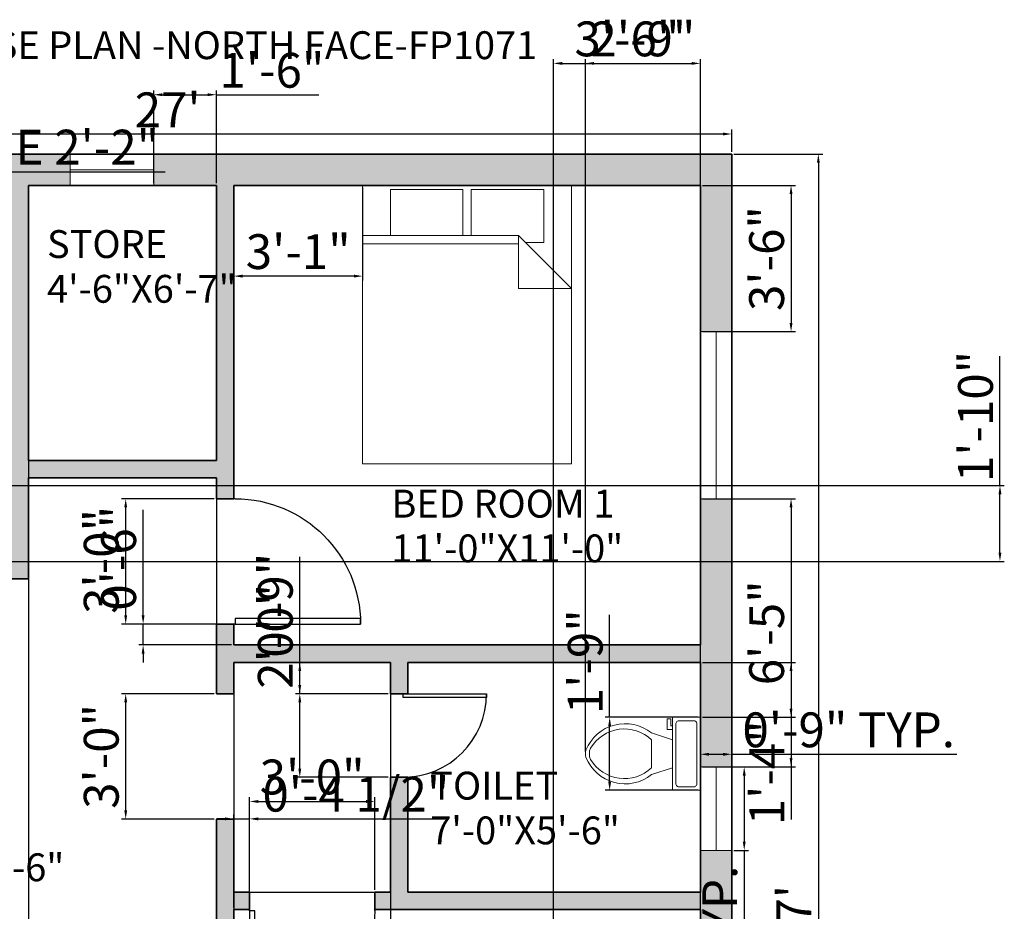
# Model space of a CAD drawing. Units: inches. Extents: x 3647 to 4124, y 1633 to 2205.
# Tile 3 of 3: x 3833 to 4116, y 1919 to 2175. Entities that reach past the tile are written whole.
import ezdxf

# ---------------------------------------------------------------- set-up
doc = ezdxf.new("R2010")
doc.units = ezdxf.units.IN
for name, color, linetype, lineweight in [('A-ANNO-DIMS', 2, 'Continuous', 18), ('A-ANNO-TEXT', 3, 'Continuous', 25), ('A-AREA-IDEN', 3, 'Continuous', 18), ('A-FLOR-FIXT', 9, 'Continuous', 18), ('A-FURN', 8, 'Continuous', 18), ('DOOR', 6, 'Continuous', 25), ('WALL', 42, 'Continuous', 35), ('WINDOW', 4, 'Continuous', 18)]:
    doc.layers.add(name, color=color, linetype=linetype, lineweight=lineweight)
doc.layers.add('A-WALL-PATT', color=18, linetype='Continuous', lineweight=13, true_color=0x000000)
doc.styles.get("Standard").update_dxf_attribs({"font": 'arial.ttf'})
doc.dimstyles.new('ISO-25', dxfattribs={"dimtxt": 10, "dimasz": 2.5, "dimexe": 1.25, "dimexo": 0.625, "dimtad": 1, "dimdec": 1, "dimlunit": 3, "dimtxsty": 'Standard', "dimcen": 2.5, "dimadec": 0, "dimazin": 0, "dimtfac": 1, "dimtdec": 1, "dimtmove": 0, "dimatfit": 3, "dimfxl": 1, "dimarcsym": 0})

# ---------------------------------------------------------------- blocks, each defined once
blk = doc.blocks.new('*U4')
for p, q in [((9.5, -6), (9.5, -2)), ((-8, -8.5), (-8, -8)), ((-7, -8), (-7, -9.5)), ((-4, -8), (-6, -14)), ((4, -8), (6, -14)), ((-10, -8.5), (-8, -8.5)), ((-10, -9.5), (-10, -8.5)), ((-7, -9.5), (-10, -9.5)), ((4, -14), (-4, -14))]:
    blk.add_line(p, q)
blk.add_lwpolyline([(10.5, -8), (10.5, 0), (-10.5, 0), (-10.5, -8)], close=True)
for points in [[(-9.5, -2), (-9.5, -6)], [(8.5, -1), (-8.5, -1)], [(-8.5, -7), (8.5, -7)]]:
    blk.add_lwpolyline(points)
for centre, radius, start, end in [((-8.62, -1.88), 0.884, 81.8699, 188.1301), ((8.62, -1.88), 0.884, 351.8699, 98.1301), ((-8.62, -6.12), 0.884, 171.8699, 278.1301), ((8.62, -6.12), 0.884, 261.8699, 8.1301), ((3.52, -21.58), 12.17, 141.4691, 247.9714), ((4.2, -21.82), 11.33, 136.3677, 238.9468), ((-3.52, -21.58), 12.17, 292.0284, 38.5307), ((-4.2, -21.82), 11.33, 301.053, 43.6321), ((0, -27.88), 4, 245.7318, 294.2682), ((0, -29), 4, 254.8605, 285.1395)]:
    blk.add_arc(centre, radius, start, end)
blk = doc.blocks.new('Bed - Queen')
for p, q in [((0, -80.00003), (0, 0)), ((0, 0), (59.99999, 0)), ((59.99999, 0), (59.99999, -80.00003)), ((7.99999, -1.2), (28.79998, -1.2)), ((7.99999, -14.4), (7.99999, -1.2)), ((28.79998, -1.2), (28.79998, -14.4)), ((31.19999, -1.2), (51.99999, -1.2)), ((31.19999, -14.4), (31.19999, -1.2)), ((51.99999, -1.2), (51.99999, -16.4)), ((0, -14.4), (44.8, -14.4)), ((44.8, -16.8), (0, -16.8)), ((59.99999, -29.6), (44.8, -14.4)), ((44.8, -14.4), (44.8, -29.6)), ((51.99999, -16.4), (46.79936, -16.4)), ((44.8, -29.6), (59.99999, -29.6)), ((59.99999, -80.00003), (0, -80.00003))]:
    blk.add_line(p, q)
blk = doc.blocks.new('*U2')
for p, q in [((0, 0), (0, -6)), ((40, 0), (40, -6))]:
    blk.add_line(p, q)
blk.add_lwpolyline([(0, 0), (0, 40), (1.75, 40), (1.75, 0)], close=True)
blk.add_arc((0, 0), 40, 0, 90)
blk = doc.blocks.new('*D11')
at = {"layer": 'A-ANNO-DIMS', "color": 0, "lineweight": -2, "transparency": 16777216}
for p, q in [((3713.71, 2136.91), (3713.71, 2143.3)), ((3716.21, 2142.05), (4035.21, 2142.05)), ((4037.71, 2136.91), (4037.71, 2143.3))]:
    blk.add_line(p, q, dxfattribs=at)
at = {"layer": 'A-ANNO-DIMS', "color": 0, "transparency": 16777216}
for points in [[(3716.21, 2142.46), (3716.21, 2141.63), (3713.71, 2142.05)], [(4035.21, 2142.46), (4035.21, 2141.63), (4037.71, 2142.05)]]:
    blk.add_solid(points, dxfattribs=at)
at = {"layer": 'Defpoints', "color": 0, "transparency": 16777216}
for p in [(4037.71, 2142.05), (3713.71, 2136.28), (4037.71, 2136.28)]:
    blk.add_point(p, dxfattribs=at)
at = {"layer": 'A-ANNO-DIMS', "color": 0, "transparency": 16777216, "insert": (3875.71, 2147.69), "char_height": 10, "attachment_point": 5}
blk.add_mtext("27'", dxfattribs=at)
blk = doc.blocks.new('*D12')
at = {"layer": 'A-ANNO-DIMS', "color": 0, "lineweight": -2, "transparency": 16777216}
for p, q in [((4038.34, 2136.28), (4063.86, 2136.28)), ((4062.61, 2133.78), (4062.61, 1694.78)), ((4038.34, 1692.28), (4063.86, 1692.28))]:
    blk.add_line(p, q, dxfattribs=at)
at = {"layer": 'A-ANNO-DIMS', "color": 0, "transparency": 16777216}
for points in [[(4062.19, 2133.78), (4063.02, 2133.78), (4062.61, 2136.28)], [(4062.19, 1694.78), (4063.02, 1694.78), (4062.61, 1692.28)]]:
    blk.add_solid(points, dxfattribs=at)
at = {"layer": 'Defpoints', "color": 0, "transparency": 16777216}
for p in [(4037.71, 2136.28), (4037.71, 1692.28), (4062.61, 1692.28)]:
    blk.add_point(p, dxfattribs=at)
at = {"layer": 'A-ANNO-DIMS', "color": 0, "transparency": 16777216, "insert": (4056.87, 1916.88), "char_height": 10, "attachment_point": 5, "rotation": 90}
blk.add_mtext("37'", dxfattribs=at)
blk = doc.blocks.new('WIN-48IN')
for p, q in [((9, 48), (0, 48)), ((4.5, 48), (4.5, 0)), ((9, 0), (0, 0))]:
    blk.add_line(p, q)
blk = doc.blocks.new('WIN-24IN')
for p, q in [((0, 0), (0, 9)), ((24, 0), (24, 9)), ((0, 4.5), (24, 4.5))]:
    blk.add_line(p, q)
blk = doc.blocks.new('*D17')
at = {"layer": 'A-ANNO-DIMS', "color": 0, "lineweight": -2, "transparency": 16777216}
for p, q in [((4038.34, 1960.28), (4042.56, 1960.28)), ((4041.31, 1957.78), (4041.31, 1938.78)), ((4038.34, 1936.28), (4042.56, 1936.28)), ((4041.31, 1936.28), (4041.31, 1836.25))]:
    blk.add_line(p, q, dxfattribs=at)
at = {"layer": 'A-ANNO-DIMS', "color": 0, "transparency": 16777216}
for points in [[(4040.9, 1957.78), (4041.73, 1957.78), (4041.31, 1960.28)], [(4040.9, 1938.78), (4041.73, 1938.78), (4041.31, 1936.28)]]:
    blk.add_solid(points, dxfattribs=at)
at = {"layer": 'Defpoints', "color": 0, "transparency": 16777216}
for p in [(4037.71, 1960.28), (4037.71, 1936.28), (4041.31, 1936.28)]:
    blk.add_point(p, dxfattribs=at)
at = {"layer": 'A-ANNO-DIMS', "color": 0, "transparency": 16777216, "insert": (4035.58, 1885.02), "char_height": 10, "attachment_point": 5, "rotation": 90}
blk.add_mtext('WIN. 2\'-0" TYP.', dxfattribs=at)
blk = doc.blocks.new('*D18')
at = {"layer": 'A-ANNO-DIMS', "color": 0, "lineweight": -2, "transparency": 16777216}
for p, q in [((4028.71, 1960.91), (4028.71, 1965.13)), ((4031.21, 1963.88), (4035.21, 1963.88)), ((4037.71, 1960.91), (4037.71, 1965.13)), ((4037.71, 1963.88), (4102.42, 1963.88))]:
    blk.add_line(p, q, dxfattribs=at)
at = {"layer": 'A-ANNO-DIMS', "color": 0, "transparency": 16777216}
for points in [[(4031.21, 1964.3), (4031.21, 1963.46), (4028.71, 1963.88)], [(4035.21, 1964.3), (4035.21, 1963.46), (4037.71, 1963.88)]]:
    blk.add_solid(points, dxfattribs=at)
at = {"layer": 'Defpoints', "color": 0, "transparency": 16777216}
for p in [(4037.71, 1963.88), (4028.71, 1960.28), (4037.71, 1960.28)]:
    blk.add_point(p, dxfattribs=at)
at = {"layer": 'A-ANNO-DIMS', "color": 0, "transparency": 16777216, "insert": (4071.32, 1969.61), "char_height": 10, "attachment_point": 5}
blk.add_mtext('0\'-9" TYP.', dxfattribs=at)
blk = doc.blocks.new('*D21')
at = {"layer": 'A-ANNO-DIMS', "color": 0, "lineweight": -2, "transparency": 16777216}
for p, q in [((3765.61, 2127.91), (3765.61, 2132.43)), ((3791.61, 2127.91), (3791.61, 2132.43)), ((3768.11, 2131.18), (3789.11, 2131.18)), ((3791.61, 2131.18), (3874.98, 2131.18))]:
    blk.add_line(p, q, dxfattribs=at)
at = {"layer": 'A-ANNO-DIMS', "color": 0, "transparency": 16777216}
for points in [[(3768.11, 2131.6), (3768.11, 2130.76), (3765.61, 2131.18)], [(3789.11, 2131.6), (3789.11, 2130.76), (3791.61, 2131.18)]]:
    blk.add_solid(points, dxfattribs=at)
at = {"layer": 'Defpoints', "color": 0, "transparency": 16777216}
for p in [(3791.61, 2131.18), (3765.61, 2127.28), (3791.61, 2127.28)]:
    blk.add_point(p, dxfattribs=at)
at = {"layer": 'A-ANNO-DIMS', "color": 0, "transparency": 16777216, "insert": (3834.55, 2136.98), "char_height": 10, "attachment_point": 5}
blk.add_mtext('RANGE 2\'-2"', dxfattribs=at)
blk = doc.blocks.new('*D25')
at = {"layer": 'A-ANNO-DIMS', "color": 0, "lineweight": -2, "transparency": 16777216}
for p, q in [((3889.09, 2037.28), (3862.41, 2037.28)), ((3863.66, 2003.78), (3863.66, 2034.78)), ((3889.09, 2001.28), (3862.41, 2001.28))]:
    blk.add_line(p, q, dxfattribs=at)
at = {"layer": 'A-ANNO-DIMS', "color": 0, "transparency": 16777216}
for points in [[(3863.25, 2034.78), (3864.08, 2034.78), (3863.66, 2037.28)], [(3863.25, 2003.78), (3864.08, 2003.78), (3863.66, 2001.28)]]:
    blk.add_solid(points, dxfattribs=at)
at = {"layer": 'Defpoints', "color": 0, "transparency": 16777216}
for p in [(3863.66, 2037.28), (3889.71, 2037.28), (3889.71, 2001.28)]:
    blk.add_point(p, dxfattribs=at)
at = {"layer": 'A-ANNO-DIMS', "color": 0, "transparency": 16777216, "insert": (3857.93, 2019.28), "char_height": 10, "attachment_point": 5, "rotation": 90}
blk.add_mtext('3\'-0"', dxfattribs=at)
blk = doc.blocks.new('*D26')
at = {"layer": 'A-ANNO-DIMS', "color": 0, "lineweight": -2, "transparency": 16777216}
for p, q in [((3913.66, 1981.28), (3913.66, 2011.78)), ((3939.09, 1981.28), (3912.41, 1981.28)), ((3913.66, 1959.78), (3913.66, 1978.78)), ((3939.09, 1957.28), (3912.41, 1957.28))]:
    blk.add_line(p, q, dxfattribs=at)
at = {"layer": 'A-ANNO-DIMS', "color": 0, "transparency": 16777216}
for points in [[(3913.25, 1978.78), (3914.08, 1978.78), (3913.66, 1981.28)], [(3913.25, 1959.78), (3914.08, 1959.78), (3913.66, 1957.28)]]:
    blk.add_solid(points, dxfattribs=at)
at = {"layer": 'Defpoints', "color": 0, "transparency": 16777216}
for p in [(3913.66, 1981.28), (3939.71, 1981.28), (3939.71, 1957.28)]:
    blk.add_point(p, dxfattribs=at)
at = {"layer": 'A-ANNO-DIMS', "color": 0, "transparency": 16777216, "insert": (3907.93, 1997.78), "char_height": 10, "attachment_point": 5, "rotation": 90}
blk.add_mtext('2\'-0"', dxfattribs=at)
blk = doc.blocks.new('*D27')
at = {"layer": 'A-ANNO-DIMS', "color": 0, "lineweight": -2, "transparency": 16777216}
for p, q in [((3899.21, 1924.91), (3899.21, 1951.58)), ((3935.21, 1924.91), (3935.21, 1951.58)), ((3901.71, 1950.33), (3932.71, 1950.33))]:
    blk.add_line(p, q, dxfattribs=at)
at = {"layer": 'A-ANNO-DIMS', "color": 0, "transparency": 16777216}
for points in [[(3901.71, 1950.75), (3901.71, 1949.91), (3899.21, 1950.33)], [(3932.71, 1950.75), (3932.71, 1949.91), (3935.21, 1950.33)]]:
    blk.add_solid(points, dxfattribs=at)
at = {"layer": 'Defpoints', "color": 0, "transparency": 16777216}
for p in [(3935.21, 1950.33), (3899.21, 1924.28), (3935.21, 1924.28)]:
    blk.add_point(p, dxfattribs=at)
at = {"layer": 'A-ANNO-DIMS', "color": 0, "transparency": 16777216, "insert": (3917.21, 1956.07), "char_height": 10, "attachment_point": 5}
blk.add_mtext('3\'-0"', dxfattribs=at)
blk = doc.blocks.new('*D29')
at = {"layer": 'A-ANNO-DIMS', "color": 0, "lineweight": -2, "transparency": 16777216}
for p, q in [((3889.09, 1981.28), (3862.41, 1981.28)), ((3863.66, 1947.78), (3863.66, 1978.78)), ((3889.09, 1945.28), (3862.41, 1945.28))]:
    blk.add_line(p, q, dxfattribs=at)
at = {"layer": 'A-ANNO-DIMS', "color": 0, "transparency": 16777216}
for points in [[(3863.25, 1978.78), (3864.08, 1978.78), (3863.66, 1981.28)], [(3863.25, 1947.78), (3864.08, 1947.78), (3863.66, 1945.28)]]:
    blk.add_solid(points, dxfattribs=at)
at = {"layer": 'Defpoints', "color": 0, "transparency": 16777216}
for p in [(3863.66, 1981.28), (3889.71, 1981.28), (3889.71, 1945.28)]:
    blk.add_point(p, dxfattribs=at)
at = {"layer": 'A-ANNO-DIMS', "color": 0, "transparency": 16777216, "insert": (3857.93, 1963.28), "char_height": 10, "attachment_point": 5, "rotation": 90}
blk.add_mtext('3\'-0"', dxfattribs=at)
blk = doc.blocks.new('*D30')
at = {"layer": 'A-ANNO-DIMS', "color": 0, "lineweight": -2, "transparency": 16777216}
for p, q in [((3894.71, 1989.66), (3894.71, 1644.98)), ((3939.71, 1989.66), (3939.71, 1644.98)), ((3897.21, 1646.23), (3937.21, 1646.23))]:
    blk.add_line(p, q, dxfattribs=at)
at = {"layer": 'A-ANNO-DIMS', "color": 0, "transparency": 16777216}
for points in [[(3897.21, 1646.65), (3897.21, 1645.81), (3894.71, 1646.23)], [(3937.21, 1646.65), (3937.21, 1645.81), (3939.71, 1646.23)]]:
    blk.add_solid(points, dxfattribs=at)
at = {"layer": 'Defpoints', "color": 0, "transparency": 16777216}
for p in [(3894.71, 1990.28), (3939.71, 1990.28), (3939.71, 1646.23)]:
    blk.add_point(p, dxfattribs=at)
at = {"layer": 'A-ANNO-DIMS', "color": 0, "transparency": 16777216, "insert": (3917.21, 1651.97), "char_height": 10, "attachment_point": 5}
blk.add_mtext('3\'-9"', dxfattribs=at)
blk = doc.blocks.new('*D32')
at = {"layer": 'A-ANNO-DIMS', "color": 0, "lineweight": -2, "transparency": 16777216}
for p, q in [((3830.71, 2126.66), (3830.71, 1644.98)), ((3835.71, 2126.66), (3835.71, 1644.98)), ((3828.21, 1646.23), (3825.71, 1646.23)), ((3830.71, 1646.23), (3835.71, 1646.23)), ((3838.21, 1646.23), (3868.55, 1646.23))]:
    blk.add_line(p, q, dxfattribs=at)
at = {"layer": 'A-ANNO-DIMS', "color": 0, "transparency": 16777216}
for points in [[(3828.21, 1646.65), (3828.21, 1645.81), (3830.71, 1646.23)], [(3838.21, 1646.65), (3838.21, 1645.81), (3835.71, 1646.23)]]:
    blk.add_solid(points, dxfattribs=at)
at = {"layer": 'Defpoints', "color": 0, "transparency": 16777216}
for p in [(3830.71, 2127.28), (3835.71, 2127.28), (3835.71, 1646.23)]:
    blk.add_point(p, dxfattribs=at)
at = {"layer": 'A-ANNO-DIMS', "color": 0, "transparency": 16777216, "insert": (3854.63, 1651.96), "char_height": 10, "attachment_point": 5}
blk.add_mtext('0\'-5"', dxfattribs=at)
blk = doc.blocks.new('*D41')
at = {"layer": 'A-ANNO-DIMS', "color": 0, "lineweight": -2, "transparency": 16777216}
for p, q in [((3871.71, 2127.91), (3871.71, 2154.58)), ((3874.21, 2153.33), (3887.21, 2153.33)), ((3889.71, 2127.91), (3889.71, 2154.58)), ((3889.71, 2153.33), (3919.1, 2153.33))]:
    blk.add_line(p, q, dxfattribs=at)
at = {"layer": 'A-ANNO-DIMS', "color": 0, "transparency": 16777216}
for points in [[(3874.21, 2153.75), (3874.21, 2152.91), (3871.71, 2153.33)], [(3887.21, 2153.75), (3887.21, 2152.91), (3889.71, 2153.33)]]:
    blk.add_solid(points, dxfattribs=at)
at = {"layer": 'Defpoints', "color": 0, "transparency": 16777216}
for p in [(3889.71, 2153.33), (3871.71, 2127.28), (3889.71, 2127.28)]:
    blk.add_point(p, dxfattribs=at)
at = {"layer": 'A-ANNO-DIMS', "color": 0, "transparency": 16777216, "insert": (3905.66, 2159.06), "char_height": 10, "attachment_point": 5}
blk.add_mtext('1\'-6"', dxfattribs=at)
blk = doc.blocks.new('*D42')
at = {"layer": 'A-ANNO-DIMS', "color": 0, "lineweight": -2, "transparency": 16777216}
for p, q in [((4029.34, 2127.28), (4056.01, 2127.28)), ((4054.76, 2124.78), (4054.76, 2087.78)), ((4029.34, 2085.28), (4056.01, 2085.28))]:
    blk.add_line(p, q, dxfattribs=at)
at = {"layer": 'A-ANNO-DIMS', "color": 0, "transparency": 16777216}
for points in [[(4054.35, 2124.78), (4055.18, 2124.78), (4054.76, 2127.28)], [(4054.35, 2087.78), (4055.18, 2087.78), (4054.76, 2085.28)]]:
    blk.add_solid(points, dxfattribs=at)
at = {"layer": 'Defpoints', "color": 0, "transparency": 16777216}
for p in [(4028.71, 2127.28), (4028.71, 2085.28), (4054.76, 2085.28)]:
    blk.add_point(p, dxfattribs=at)
at = {"layer": 'A-ANNO-DIMS', "color": 0, "transparency": 16777216, "insert": (4049.03, 2106.28), "char_height": 10, "attachment_point": 5, "rotation": 90}
blk.add_mtext('3\'-6"', dxfattribs=at)
blk = doc.blocks.new('*D43')
at = {"layer": 'A-ANNO-DIMS', "color": 0, "lineweight": -2, "transparency": 16777216}
for p, q in [((4029.34, 2037.28), (4056.01, 2037.28)), ((4054.76, 2034.78), (4054.76, 1962.78)), ((4029.34, 1960.28), (4056.01, 1960.28))]:
    blk.add_line(p, q, dxfattribs=at)
at = {"layer": 'A-ANNO-DIMS', "color": 0, "transparency": 16777216}
for points in [[(4054.35, 2034.78), (4055.18, 2034.78), (4054.76, 2037.28)], [(4054.35, 1962.78), (4055.18, 1962.78), (4054.76, 1960.28)]]:
    blk.add_solid(points, dxfattribs=at)
at = {"layer": 'Defpoints', "color": 0, "transparency": 16777216}
for p in [(4028.71, 2037.28), (4028.71, 1960.28), (4054.76, 1960.28)]:
    blk.add_point(p, dxfattribs=at)
at = {"layer": 'A-ANNO-DIMS', "color": 0, "transparency": 16777216, "insert": (4049.03, 1998.78), "char_height": 10, "attachment_point": 5, "rotation": 90}
blk.add_mtext('6\'-5"', dxfattribs=at)
blk = doc.blocks.new('*D48')
at = {"layer": 'A-ANNO-DIMS', "color": 0, "lineweight": -2, "transparency": 16777216}
for p, q in [((3868.66, 2003.78), (3868.66, 2034.11)), ((3894.09, 2001.28), (3867.41, 2001.28)), ((3868.66, 1995.28), (3868.66, 2001.28)), ((3894.09, 1995.28), (3867.41, 1995.28)), ((3868.66, 1992.78), (3868.66, 1990.28))]:
    blk.add_line(p, q, dxfattribs=at)
at = {"layer": 'A-ANNO-DIMS', "color": 0, "transparency": 16777216}
for points in [[(3868.25, 2003.78), (3869.08, 2003.78), (3868.66, 2001.28)], [(3868.25, 1992.78), (3869.08, 1992.78), (3868.66, 1995.28)]]:
    blk.add_solid(points, dxfattribs=at)
at = {"layer": 'Defpoints', "color": 0, "transparency": 16777216}
for p in [(3868.66, 2001.28), (3894.71, 2001.28), (3894.71, 1995.28)]:
    blk.add_point(p, dxfattribs=at)
at = {"layer": 'A-ANNO-DIMS', "color": 0, "transparency": 16777216, "insert": (3862.93, 2020.2), "char_height": 10, "attachment_point": 5, "rotation": 90}
blk.add_mtext('0\'-6"', dxfattribs=at)
blk = doc.blocks.new('*D49')
at = {"layer": 'A-ANNO-DIMS', "color": 0, "lineweight": -2, "transparency": 16777216}
for p, q in [((3894.71, 1919.91), (3894.71, 1946.58)), ((3899.21, 1919.91), (3899.21, 1946.58)), ((3892.21, 1945.33), (3889.71, 1945.33)), ((3894.71, 1945.33), (3899.21, 1945.33)), ((3901.71, 1945.33), (3955.35, 1945.33))]:
    blk.add_line(p, q, dxfattribs=at)
at = {"layer": 'A-ANNO-DIMS', "color": 0, "transparency": 16777216}
for points in [[(3892.21, 1945.75), (3892.21, 1944.91), (3894.71, 1945.33)], [(3901.71, 1945.75), (3901.71, 1944.91), (3899.21, 1945.33)]]:
    blk.add_solid(points, dxfattribs=at)
at = {"layer": 'Defpoints', "color": 0, "transparency": 16777216}
for p in [(3899.21, 1945.33), (3894.71, 1919.28), (3899.21, 1919.28)]:
    blk.add_point(p, dxfattribs=at)
at = {"layer": 'A-ANNO-DIMS', "color": 0, "transparency": 16777216, "insert": (3929.78, 1951.13), "char_height": 10, "attachment_point": 5}
blk.add_mtext('0\'-4 1/2"', dxfattribs=at)
blk = doc.blocks.new('*D50')
at = {"layer": 'A-ANNO-DIMS', "color": 0, "lineweight": -2, "transparency": 16777216}
for p, q in [((3913.66, 1990.28), (3913.66, 2020.61)), ((3939.09, 1990.28), (3912.41, 1990.28)), ((3913.66, 1983.78), (3913.66, 1987.78)), ((3939.09, 1981.28), (3912.41, 1981.28))]:
    blk.add_line(p, q, dxfattribs=at)
at = {"layer": 'A-ANNO-DIMS', "color": 0, "transparency": 16777216}
for points in [[(3913.25, 1987.78), (3914.08, 1987.78), (3913.66, 1990.28)], [(3913.25, 1983.78), (3914.08, 1983.78), (3913.66, 1981.28)]]:
    blk.add_solid(points, dxfattribs=at)
at = {"layer": 'Defpoints', "color": 0, "transparency": 16777216}
for p in [(3913.66, 1990.28), (3939.71, 1990.28), (3939.71, 1981.28)]:
    blk.add_point(p, dxfattribs=at)
at = {"layer": 'A-ANNO-DIMS', "color": 0, "transparency": 16777216, "insert": (3907.93, 2006.7), "char_height": 10, "attachment_point": 5, "rotation": 90}
blk.add_mtext('0\'-9"', dxfattribs=at)
blk = doc.blocks.new('*D55')
at = {"layer": 'A-ANNO-DIMS', "color": 0, "lineweight": -2, "transparency": 16777216}
for p, q in [((4114.76, 2041.09), (4114.76, 2078.26)), ((3744.18, 2041.09), (4116.01, 2041.09)), ((4114.76, 2021.78), (4114.76, 2038.59)), ((3747.34, 2019.28), (4116.01, 2019.28))]:
    blk.add_line(p, q, dxfattribs=at)
at = {"layer": 'A-ANNO-DIMS', "color": 0, "transparency": 16777216}
for points in [[(4114.35, 2038.59), (4115.18, 2038.59), (4114.76, 2041.09)], [(4114.35, 2021.78), (4115.18, 2021.78), (4114.76, 2019.28)]]:
    blk.add_solid(points, dxfattribs=at)
at = {"layer": 'Defpoints', "color": 0, "transparency": 16777216}
for p in [(3743.56, 2041.09), (4114.76, 2041.09), (3746.71, 2019.28)]:
    blk.add_point(p, dxfattribs=at)
at = {"layer": 'A-ANNO-DIMS', "color": 0, "transparency": 16777216, "insert": (4109.03, 2060.92), "char_height": 10, "attachment_point": 5, "rotation": 90}
blk.add_mtext('1\'-10"', dxfattribs=at)
blk = doc.blocks.new('*D56')
at = {"layer": 'A-ANNO-DIMS', "color": 0, "lineweight": -2, "transparency": 16777216}
for p, q in [((4029.34, 1990.28), (4056.01, 1990.28)), ((4054.76, 1987.78), (4054.76, 1977.03)), ((4029.34, 1974.53), (4056.01, 1974.53)), ((4054.76, 1974.53), (4054.76, 1945.14))]:
    blk.add_line(p, q, dxfattribs=at)
at = {"layer": 'A-ANNO-DIMS', "color": 0, "transparency": 16777216}
for points in [[(4054.35, 1987.78), (4055.18, 1987.78), (4054.76, 1990.28)], [(4054.35, 1977.03), (4055.18, 1977.03), (4054.76, 1974.53)]]:
    blk.add_solid(points, dxfattribs=at)
at = {"layer": 'Defpoints', "color": 0, "transparency": 16777216}
for p in [(4028.71, 1990.28), (4028.71, 1974.53), (4054.76, 1974.53)]:
    blk.add_point(p, dxfattribs=at)
at = {"layer": 'A-ANNO-DIMS', "color": 0, "transparency": 16777216, "insert": (4049.12, 1958.58), "char_height": 10, "attachment_point": 5, "rotation": 90}
blk.add_mtext('1\'-4"', dxfattribs=at)
blk = doc.blocks.new('*D57')
at = {"layer": 'A-ANNO-DIMS', "color": 0, "lineweight": -2, "transparency": 16777216}
for p, q in [((4002.66, 1974.53), (4002.66, 2003.92)), ((4028.09, 1974.53), (4001.41, 1974.53)), ((4002.66, 1956.03), (4002.66, 1972.03)), ((4028.09, 1953.53), (4001.41, 1953.53))]:
    blk.add_line(p, q, dxfattribs=at)
at = {"layer": 'A-ANNO-DIMS', "color": 0, "transparency": 16777216}
for points in [[(4002.25, 1972.03), (4003.08, 1972.03), (4002.66, 1974.53)], [(4002.25, 1956.03), (4003.08, 1956.03), (4002.66, 1953.53)]]:
    blk.add_solid(points, dxfattribs=at)
at = {"layer": 'Defpoints', "color": 0, "transparency": 16777216}
for p in [(4002.66, 1974.53), (4028.71, 1974.53), (4028.71, 1953.53)]:
    blk.add_point(p, dxfattribs=at)
at = {"layer": 'A-ANNO-DIMS', "color": 0, "transparency": 16777216, "insert": (3996.93, 1990.48), "char_height": 10, "attachment_point": 5, "rotation": 90}
blk.add_mtext('1\'-9"', dxfattribs=at)
blk = doc.blocks.new('*D58')
at = {"layer": 'A-ANNO-DIMS', "color": 0, "lineweight": -2, "transparency": 16777216}
for p, q in [((3995.71, 1964.65), (3995.71, 2163.58)), ((4028.71, 1975.15), (4028.71, 2163.58)), ((3998.21, 2162.33), (4026.21, 2162.33))]:
    blk.add_line(p, q, dxfattribs=at)
at = {"layer": 'A-ANNO-DIMS', "color": 0, "transparency": 16777216}
for points in [[(3998.21, 2162.75), (3998.21, 2161.91), (3995.71, 2162.33)], [(4026.21, 2162.75), (4026.21, 2161.91), (4028.71, 2162.33)]]:
    blk.add_solid(points, dxfattribs=at)
at = {"layer": 'Defpoints', "color": 0, "transparency": 16777216}
for p in [(4028.71, 2162.33), (4028.71, 1974.53), (3995.71, 1964.03)]:
    blk.add_point(p, dxfattribs=at)
at = {"layer": 'A-ANNO-DIMS', "color": 0, "transparency": 16777216, "insert": (4012.21, 2168.06), "char_height": 10, "attachment_point": 5}
blk.add_mtext('2\'-9"', dxfattribs=at)
blk = doc.blocks.new('*D59')
at = {"layer": 'A-ANNO-DIMS', "color": 0, "lineweight": -2, "transparency": 16777216}
for p, q in [((3894.71, 2126.66), (3894.71, 2099.98)), ((3931.71, 2126.66), (3931.71, 2099.98)), ((3929.21, 2101.23), (3897.21, 2101.23))]:
    blk.add_line(p, q, dxfattribs=at)
at = {"layer": 'A-ANNO-DIMS', "color": 0, "transparency": 16777216}
for points in [[(3897.21, 2101.65), (3897.21, 2100.81), (3894.71, 2101.23)], [(3929.21, 2101.65), (3929.21, 2100.81), (3931.71, 2101.23)]]:
    blk.add_solid(points, dxfattribs=at)
at = {"layer": 'Defpoints', "color": 0, "transparency": 16777216}
for p in [(3894.71, 2127.28), (3931.71, 2127.28), (3894.71, 2101.23)]:
    blk.add_point(p, dxfattribs=at)
at = {"layer": 'A-ANNO-DIMS', "color": 0, "transparency": 16777216, "insert": (3913.21, 2106.97), "char_height": 10, "attachment_point": 5}
blk.add_mtext('3\'-1"', dxfattribs=at)
blk = doc.blocks.new('*D60')
at = {"layer": 'A-ANNO-DIMS', "color": 0, "lineweight": -2, "transparency": 16777216}
for p, q in [((3986.53, 1784.49), (3986.53, 2163.58)), ((4028.71, 1780.91), (4028.71, 2163.58)), ((3989.03, 2162.33), (4026.21, 2162.33))]:
    blk.add_line(p, q, dxfattribs=at)
at = {"layer": 'A-ANNO-DIMS', "color": 0, "transparency": 16777216}
for points in [[(3989.03, 2162.75), (3989.03, 2161.91), (3986.53, 2162.33)], [(4026.21, 2162.75), (4026.21, 2161.91), (4028.71, 2162.33)]]:
    blk.add_solid(points, dxfattribs=at)
at = {"layer": 'Defpoints', "color": 0, "transparency": 16777216}
for p in [(4028.71, 2162.33), (3986.53, 1783.86), (4028.71, 1780.28)]:
    blk.add_point(p, dxfattribs=at)
at = {"layer": 'A-ANNO-DIMS', "color": 0, "transparency": 16777216, "insert": (4007.62, 2168.07), "char_height": 10, "attachment_point": 5}
blk.add_mtext('3\'-6"', dxfattribs=at)

msp = doc.modelspace()

# ---------------------------------------------------------------- hatches: boundary and pattern name
at = {"layer": 'A-WALL-PATT'}
h = msp.add_hatch(color=256, dxfattribs=at)
h.dxf.hatch_style = 1
h.paths.add_polyline_path([(3847.71, 2136.28), (3713.71, 2136.28), (3713.71, 2091.28), (3722.71, 2091.28), (3722.71, 2127.28), (3830.71, 2127.28), (3830.71, 2014.28), (3835.71, 2014.28), (3835.71, 2043.28), (3889.71, 2043.28), (3889.71, 2037.28), (3894.71, 2037.28), (3894.71, 2127.28), (4028.71, 2127.28), (4028.71, 2085.28), (4037.71, 2085.28), (4037.71, 2136.28), (3871.71, 2136.28), (3871.71, 2127.28), (3889.71, 2127.28), (3889.71, 2048.28), (3835.71, 2048.28), (3835.71, 2127.28), (3847.71, 2127.28)])
h.paths.add_polyline_path([(3839.02, 2091.4), (3895.07, 2091.4), (3895.07, 2103.66), (3839.02, 2103.66)], flags=25)
h = msp.add_hatch(color=256, dxfattribs=at)
h.dxf.hatch_style = 1
h.paths.add_polyline_path([(4037.71, 2037.28), (4028.71, 2037.28), (4028.71, 1995.28), (3894.71, 1995.28), (3894.71, 2001.28), (3889.71, 2001.28), (3889.71, 1981.28), (3894.71, 1981.28), (3894.71, 1990.28), (3939.71, 1990.28), (3939.71, 1981.28), (3943.31, 1981.28), (3944.71, 1981.28), (3944.71, 1990.28), (4028.71, 1990.28), (4028.71, 1960.28), (4037.71, 1960.28)])
h = msp.add_hatch(color=256, dxfattribs=at)
h.dxf.hatch_style = 1
h.paths.add_polyline_path([(4037.71, 1936.28), (4028.71, 1936.28), (4028.71, 1924.28), (3944.71, 1924.28), (3944.71, 1957.28), (3939.71, 1957.28), (3939.71, 1924.28), (3935.21, 1924.28), (3935.21, 1919.28), (4028.71, 1919.28), (4028.71, 1870.28), (4037.71, 1870.28)])
h = msp.add_hatch(color=256, dxfattribs=at)
h.dxf.hatch_style = 1
h.paths.add_polyline_path([(4037.71, 1822.28), (4028.71, 1822.28), (4028.71, 1780.28), (3894.71, 1780.28), (3894.71, 1919.28), (3899.21, 1919.28), (3899.21, 1924.28), (3894.71, 1924.28), (3894.71, 1945.28), (3889.71, 1945.28), (3889.71, 1876.28), (3880.71, 1876.28), (3880.71, 1871.28), (3889.71, 1871.28), (3889.71, 1775.28), (4028.71, 1775.28), (4028.71, 1755.28), (4037.71, 1755.28)])

# ---------------------------------------------------------------- linework, layer by layer
at = {"layer": 'DOOR'}
for p, q in [((3889.71, 2037.28), (3889.71, 2001.28)), ((3939.71, 1981.28), (3939.71, 1957.28)), ((3899.21, 1924.28), (3935.21, 1924.28))]:
    msp.add_line(p, q, dxfattribs=at)
at = {"layer": 'WALL'}
for p, q in [((3713.71, 2136.28), (4037.71, 2136.28)), ((4037.71, 2136.28), (4037.71, 1692.28)), ((3835.71, 2127.28), (3889.71, 2127.28)), ((3835.71, 2048.28), (3835.71, 2127.28)), ((3889.71, 2048.28), (3889.71, 2127.28)), ((3894.71, 2127.28), (4028.71, 2127.28)), ((3894.71, 2037.28), (3894.71, 2127.28)), ((4028.71, 2127.28), (4028.71, 1995.28)), ((3835.71, 2048.28), (3889.71, 2048.28)), ((3835.71, 2014.28), (3835.71, 2043.28)), ((3835.71, 2043.28), (3889.71, 2043.28)), ((3889.71, 2037.28), (3889.71, 2043.28)), ((3889.71, 2037.28), (3894.71, 2037.28)), ((3830.71, 2014.28), (3835.71, 2014.28)), ((3889.71, 2001.28), (3894.71, 2001.28)), ((3889.71, 1981.28), (3889.71, 2001.28)), ((3894.71, 1995.28), (3894.71, 2001.28)), ((3894.71, 1995.28), (4028.71, 1995.28)), ((3894.71, 1990.28), (3939.71, 1990.28)), ((3894.71, 1981.28), (3894.71, 1990.28)), ((3939.71, 1990.28), (3939.71, 1981.28)), ((3944.71, 1990.28), (3944.71, 1981.28)), ((3944.71, 1990.28), (4028.71, 1990.28)), ((4028.71, 1990.28), (4028.71, 1924.28)), ((3894.71, 1981.28), (3889.71, 1981.28)), ((3944.71, 1981.28), (3939.71, 1981.28)), ((3944.71, 1957.28), (3939.71, 1957.28)), ((3939.71, 1957.28), (3939.71, 1924.28)), ((3944.71, 1957.28), (3944.71, 1924.28)), ((3889.71, 1876.28), (3889.71, 1945.28)), ((3894.71, 1945.28), (3889.71, 1945.28)), ((3894.71, 1924.28), (3894.71, 1945.28)), ((3894.71, 1924.28), (3899.21, 1924.28)), ((3899.21, 1924.28), (3899.21, 1919.28)), ((3935.21, 1924.28), (3935.21, 1919.28)), ((3935.21, 1924.28), (3939.71, 1924.28)), ((3944.71, 1924.28), (4028.71, 1924.28)), ((3894.71, 1780.28), (3894.71, 1919.28)), ((3894.71, 1919.28), (3899.21, 1919.28)), ((3935.21, 1919.28), (4028.71, 1919.28)), ((4028.71, 1919.28), (4028.71, 1780.28))]:
    msp.add_line(p, q, dxfattribs=at)

# ---------------------------------------------------------------- block references
at = {"layer": 'A-FLOR-FIXT', "rotation": 270}
msp.add_blockref('*U4', (4028.71, 1964.03), dxfattribs=at)
at = {"layer": 'A-FURN'}
msp.add_blockref('Bed - Queen', (3931.71, 2127.28), dxfattribs=at)
at = {"layer": 'DOOR'}
for p, xscale, yscale, zscale, rotation in [((3895.11, 2001.28), -0.9, 0.9, 0.9, 270), ((3943.31, 1981.28), 0.6, 0.6, 0.6, 270), ((3899.21, 1918.88), -0.9, 0.9, 0.9, 180)]:
    msp.add_blockref('*U2', p, dxfattribs=dict(at, xscale=xscale, yscale=yscale, zscale=zscale, rotation=rotation))
at = {"layer": 'WINDOW'}
msp.add_blockref('WIN-24IN', (3847.71, 2127.28), dxfattribs=at)
for name, p, rotation in [('WIN-48IN', (4037.71, 2085.28), 180), ('WIN-24IN', (4028.71, 1960.28), 270.0000000000021)]:
    msp.add_blockref(name, p, dxfattribs=dict(at, rotation=rotation))

# ---------------------------------------------------------------- texts
at = {"layer": 'A-ANNO-TEXT'}
msp.add_text('27X37 (999 SQ FT) HOUSE PLAN -NORTH FACE-FP1071', height=8, dxfattribs=at).set_placement((3709.15, 2163.55))
at = {"layer": 'A-AREA-IDEN'}
for s, p in [('STORE', (3841.06, 2106.43)), ('4\'-6"X6\'-7"', (3841.06, 2093.58)), ('BED ROOM 1', (3939.98, 2031.87)), ('11\'-0"X11\'-0"', (3939.98, 2019.02)), ('TOILET', (3951.13, 1950.87)), ('7\'-0"X5\'-6"', (3951.13, 1938.02)), ('13\'-11"X11\'-6"', (3773.39, 1927.42))]:
    msp.add_text(s, height=8, dxfattribs=at).set_placement(p)

# ---------------------------------------------------------------- dimensions: what is measured, and where the dimension line sits
at = {"layer": 'A-ANNO-DIMS'}
for base, p1, p2, override, picture, middle in [((4028.71, 2162.33), (3986.53, 1783.86), (4028.71, 1780.28), {"dimdec": 1, "dimlfac": 1, "dimrnd": 0, "dimzin": 1, "dimdsep": 46, "dimlunit": 4, "dimfrac": 2}, '*D60', (4007.62, 2168.07)), ((4028.71, 2162.33), (3995.71, 1964.03), (4028.71, 1974.53), {"dimdec": 1, "dimlfac": 1, "dimrnd": 0, "dimzin": 1, "dimdsep": 46, "dimlunit": 4, "dimfrac": 2}, '*D58', (4012.21, 2168.06)), ((3889.71, 2153.33), (3871.71, 2127.28), (3889.71, 2127.28), {"dimdec": 1, "dimlfac": 1, "dimrnd": 0, "dimzin": 1, "dimdsep": 46, "dimlunit": 4, "dimfrac": 2}, '*D41', (3905.66, 2159.06)), ((4037.71, 2142.05), (3713.71, 2136.28), (4037.71, 2136.28), {"dimclrd": 0, "dimclre": 0, "dimclrt": 0}, '*D11', (3875.71, 2147.69)), ((3835.71, 1646.23), (3830.71, 2127.28), (3835.71, 2127.28), {"dimdec": 1, "dimlfac": 1, "dimrnd": 0, "dimzin": 1, "dimdsep": 46, "dimlunit": 4, "dimfrac": 2}, '*D32', (3854.63, 1651.96)), ((3939.71, 1646.23), (3894.71, 1990.28), (3939.71, 1990.28), {"dimdec": 1, "dimlfac": 1, "dimrnd": 0, "dimzin": 1, "dimdsep": 46, "dimlunit": 4, "dimfrac": 2}, '*D30', (3917.21, 1651.97)), ((3899.21, 1945.33), (3894.71, 1919.28), (3899.21, 1919.28), {"dimdec": 1, "dimlfac": 1, "dimrnd": 0, "dimzin": 1, "dimdsep": 46, "dimlunit": 4, "dimfrac": 2}, '*D49', (3929.78, 1951.13)), ((3935.21, 1950.33), (3899.21, 1924.28), (3935.21, 1924.28), {"dimdec": 1, "dimlfac": 1, "dimrnd": 0, "dimzin": 1, "dimdsep": 46, "dimlunit": 4, "dimfrac": 2}, '*D27', (3917.21, 1956.07))]:
    dim = msp.add_linear_dim(base=base, p1=p1, p2=p2, dimstyle='ISO-25', override=override, dxfattribs=at)
    dim.commit()
    dim.dimension.update_dxf_attribs({"geometry": picture, "text_midpoint": middle})
dim = msp.add_linear_dim(base=(3791.61, 2131.18), p1=(3765.61, 2127.28), p2=(3791.61, 2127.28), text='RANGE <>', dimstyle='ISO-25', override={"dimdec": 1, "dimlfac": 1, "dimrnd": 0, "dimzin": 1, "dimdsep": 46, "dimlunit": 4, "dimfrac": 2}, dxfattribs=at)
dim.commit()
dim.dimension.update_dxf_attribs({"geometry": '*D21', "text_midpoint": (3834.55, 2136.98)})
dim = msp.add_linear_dim(base=(4062.61, 1692.28), p1=(4037.71, 2136.28), p2=(4037.71, 1692.28), angle=90, dimstyle='ISO-25', override={"dimclrd": 0, "dimclre": 0, "dimclrt": 0}, dxfattribs=at)
dim.commit()
dim.dimension.update_dxf_attribs({"geometry": '*D12', "text_midpoint": (4062.61, 1916.88), "dimtype": 160})
for base, p1, p2, angle, picture, middle in [((3894.71, 2101.23), (3931.71, 2127.28), (3894.71, 2127.28), 180, '*D59', (3913.21, 2106.97)), ((4054.76, 2085.28), (4028.71, 2127.28), (4028.71, 2085.28), 270, '*D42', (4049.03, 2106.28)), ((4114.76, 2041.09), (3746.71, 2019.28), (3743.56, 2041.09), 90, '*D55', (4109.03, 2060.92)), ((3863.66, 2037.28), (3889.71, 2001.28), (3889.71, 2037.28), 90, '*D25', (3857.93, 2019.28)), ((4054.76, 1960.28), (4028.71, 2037.28), (4028.71, 1960.28), 270, '*D43', (4049.03, 1998.78)), ((3868.66, 2001.28), (3894.71, 1995.28), (3894.71, 2001.28), 90, '*D48', (3862.93, 2020.2)), ((3913.66, 1990.28), (3939.71, 1981.28), (3939.71, 1990.28), 90, '*D50', (3907.93, 2006.7)), ((3913.66, 1981.28), (3939.71, 1957.28), (3939.71, 1981.28), 90, '*D26', (3907.93, 1997.78)), ((4002.66, 1974.53), (4028.71, 1953.53), (4028.71, 1974.53), 90, '*D57', (3996.93, 1990.48)), ((4054.7637, 1974.5297), (4028.7137, 1990.2816), (4028.7137, 1974.5297), 270, '*D56', (4049.1183, 1958.5841)), ((3863.66, 1981.28), (3889.71, 1945.28), (3889.71, 1981.28), 90, '*D29', (3857.93, 1963.28))]:
    dim = msp.add_linear_dim(base=base, p1=p1, p2=p2, angle=angle, dimstyle='ISO-25', override={"dimdec": 1, "dimlfac": 1, "dimrnd": 0, "dimzin": 1, "dimdsep": 46, "dimlunit": 4, "dimfrac": 2}, dxfattribs=at)
    dim.commit()
    dim.dimension.update_dxf_attribs({"geometry": picture, "text_midpoint": middle})
for base, p1, p2, angle, text, picture, middle in [((4037.71, 1963.88), (4028.71, 1960.28), (4037.71, 1960.28), 0, '<> TYP.', '*D18', (4071.32, 1969.61)), ((4041.31, 1936.28), (4037.71, 1960.28), (4037.71, 1936.28), 270, 'WIN. <> TYP.', '*D17', (4035.58, 1885.02))]:
    dim = msp.add_linear_dim(base=base, p1=p1, p2=p2, angle=angle, text=text, dimstyle='ISO-25', override={"dimdec": 1, "dimlfac": 1, "dimrnd": 0, "dimzin": 1, "dimdsep": 46, "dimlunit": 4, "dimfrac": 2}, dxfattribs=at)
    dim.commit()
    dim.dimension.update_dxf_attribs({"geometry": picture, "text_midpoint": middle})

doc.saveas('drawing.dxf')
